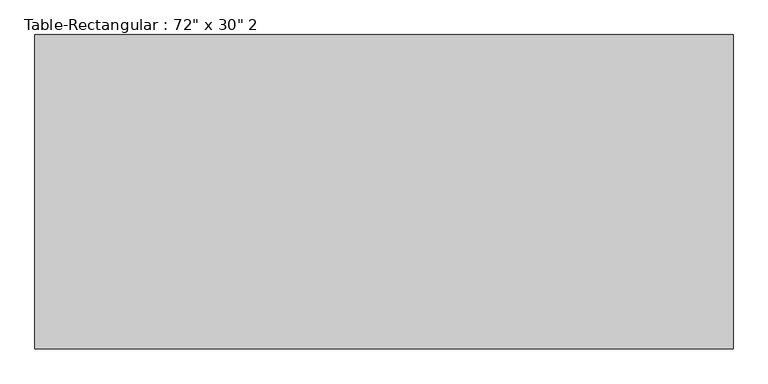
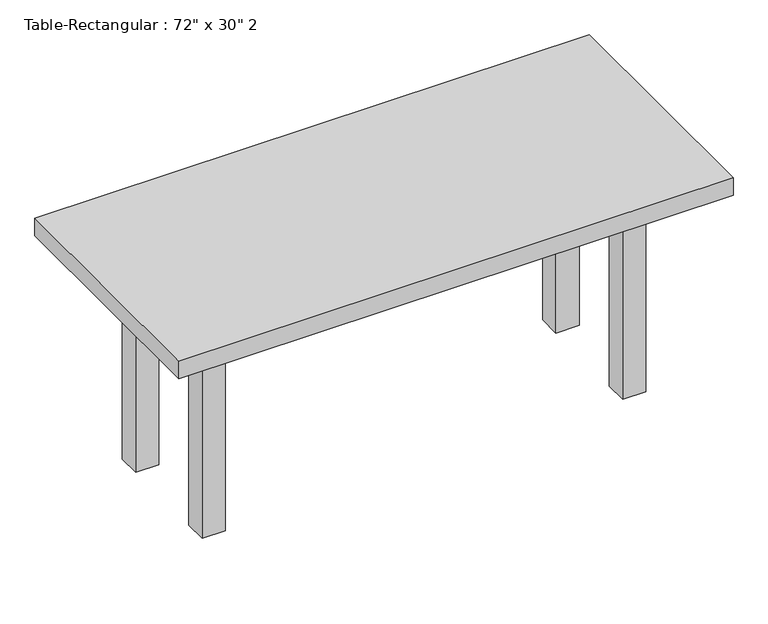
"""IFC4 building model written with IfcOpenShell, lengths in millimetres: furniture geometry."""

from ifc_helpers import new_model, si_unit, frame, origin, origin_with_axes, place, context, project, spatial, polyline, outline, extrude, source, transform, mapped, element, save


def furniture_06ea8467(model_context):
    return source(origin(), model_context, "Body", "SweptSolid", [
        extrude(outline(polyline([(546.1, 152.4), (546.1, 127.0), (-546.1, 127.0), (-546.1, 152.4), (546.1, 152.4)])), frame((0.0, 0.0, 508.0), z_axis=(0.0, 0.0, 1.0), x_axis=(1.0, 0.0, 0.0)), (0.0, 0.0, 1.0), 101.6),
        extrude(outline(polyline([(546.1, -152.4), (-546.1, -152.4), (-546.1, -127.0), (546.1, -127.0), (546.1, -152.4)])), frame((0.0, 0.0, 508.0), z_axis=(0.0, 0.0, 1.0), x_axis=(1.0, 0.0, 0.0)), (0.0, 0.0, 1.0), 101.6),
        extrude(outline(polyline([(-558.8, -127.0), (-584.2, -127.0), (-584.2, 127.0), (-558.8, 127.0), (-558.8, -127.0)])), frame((0.0, 0.0, 508.0), z_axis=(0.0, 0.0, 1.0), x_axis=(1.0, 0.0, 0.0)), (0.0, 0.0, 1.0), 101.6),
        extrude(outline(polyline([(558.8, -127.0), (558.8, 127.0), (584.2, 127.0), (584.2, -127.0), (558.8, -127.0)])), frame((0.0, 0.0, 508.0), z_axis=(0.0, 0.0, 1.0), x_axis=(1.0, 0.0, 0.0)), (0.0, 0.0, 1.0), 101.6),
        extrude(outline(polyline([(762.0, 342.9), (762.0, -342.9), (-762.0, -342.9), (-762.0, 342.9), (762.0, 342.9)])), frame((0.0, 0.0, 609.6), z_axis=(0.0, 0.0, 1.0), x_axis=(1.0, 0.0, 0.0)), (0.0, 0.0, 1.0), 50.8),
        extrude(outline(polyline([(-546.1, 190.5), (-546.1, 127.0), (-609.6, 127.0), (-609.6, 190.5), (-546.1, 190.5)])), origin_with_axes(), (0.0, 0.0, 1.0), 609.6),
        extrude(outline(polyline([(546.1, 190.5), (609.6, 190.5), (609.6, 127.0), (546.1, 127.0), (546.1, 190.5)])), origin_with_axes(), (0.0, 0.0, 1.0), 609.6),
        extrude(outline(polyline([(-546.1, -190.5), (-609.6, -190.5), (-609.6, -127.0), (-546.1, -127.0), (-546.1, -190.5)])), origin_with_axes(), (0.0, 0.0, 1.0), 609.6),
        extrude(outline(polyline([(546.1, -190.5), (546.1, -127.0), (609.6, -127.0), (609.6, -190.5), (546.1, -190.5)])), origin_with_axes(), (0.0, 0.0, 1.0), 609.6),
    ])


if __name__ == "__main__":
    model = new_model("IFC4")
    model_context = context("Model", 3, world=origin())
    ifc_project = project(units=[si_unit("LENGTHUNIT", "METRE", prefix="MILLI")], contexts=[model_context])
    site = spatial("IfcSite", under=ifc_project)
    building = spatial("IfcBuilding", under=site)
    placement = place(None, origin())
    furniture_shape = furniture_06ea8467(model_context)
    element("IfcFurniture", 1, ObjectType="Table-Rectangular : 72\" x 30\" 2", at=placement, inside=building, context=model_context, shape_type="MappedRepresentation", body=[
        mapped(furniture_shape, transform((0.0, 0.0, 0.0), x_axis=(1.0, 0.0, 0.0), y_axis=(0.0, 1.0, 0.0), z_axis=(0.0, 0.0, 1.0))),
    ])
    save(model, "model.ifc")

# Revit data of these elements
# Type "Table-Rectangular : 72\" x 30\" 2"
#   Assembly Code = "E2020200"
#   Height = 2' - 2"
#   Length = 5' - 0"
#   Width = 2' - 3"
#   Base Material = Birch
#   Top Material = Birch
#   Default Elevation = 0
# Element 1 (IfcFurniture, "Table-Rectangular : 72\" x 30\" 2")
#   Materials on its faces: "Birch"
# Materials
#   "Birch": class "Wood", colour RGB 224 178 126, transparency 0, Description = "Betula Alleghaniensis", Cost = 0
